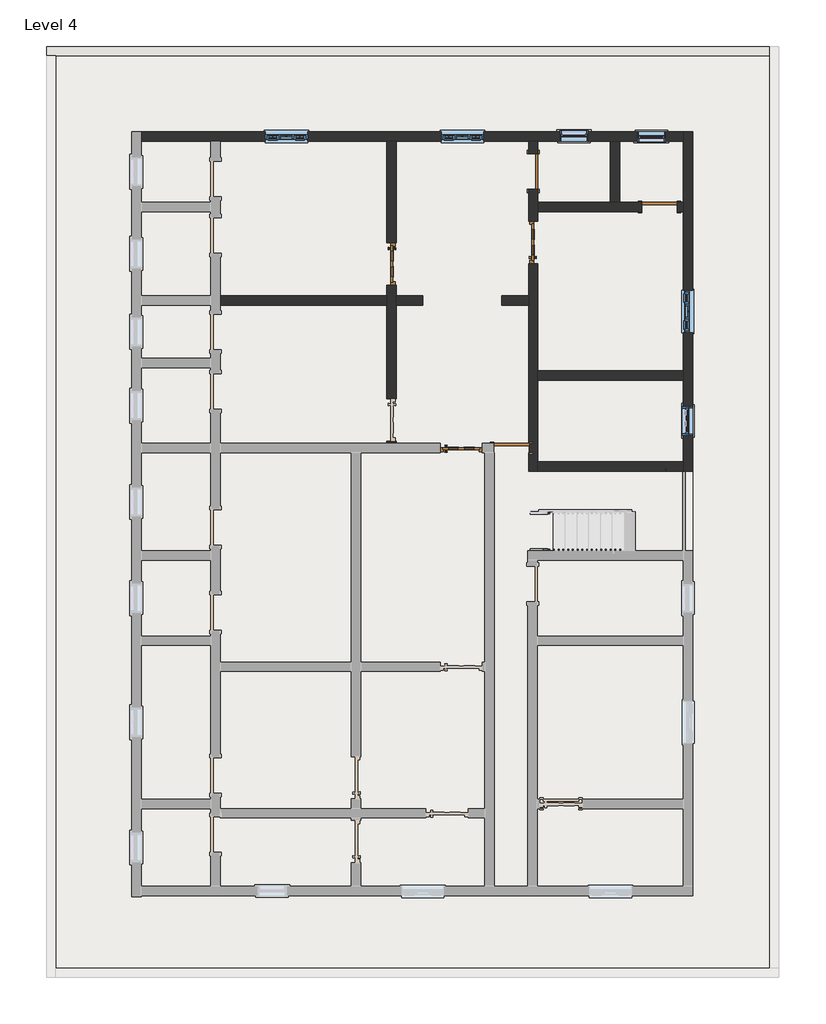
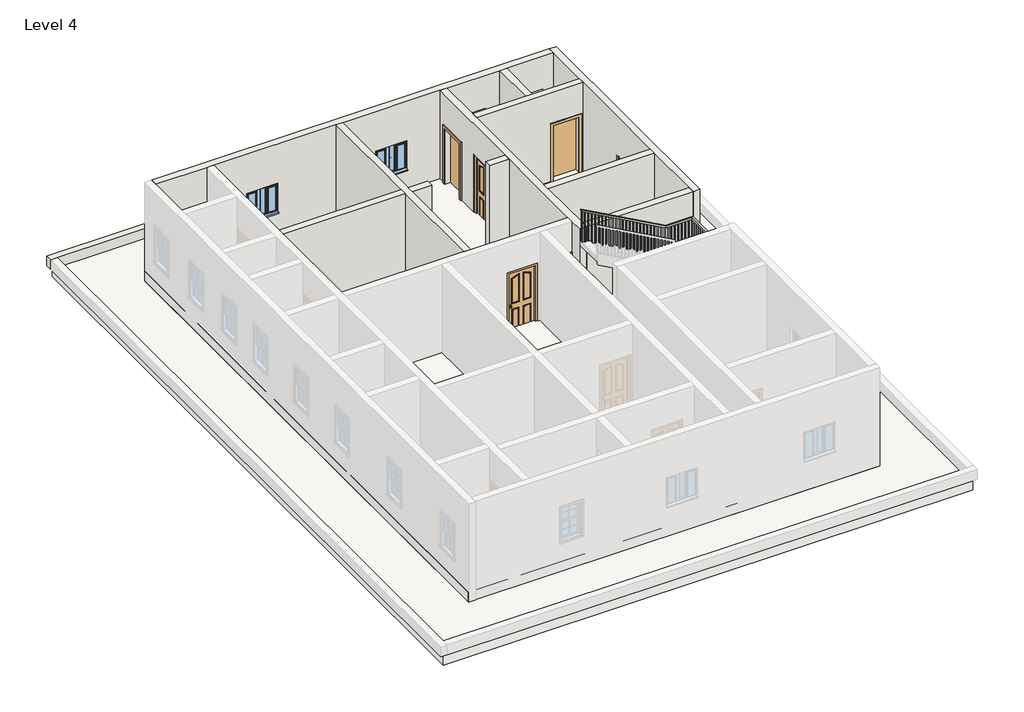
# One storey, part 2 of 3: 11 walls, 6 doors, 6 windows, 2 slabs, 1 railing, 1 roof.
"""IFC4 building model written with IfcOpenShell, lengths in millimetres."""

from ifc_helpers import new_model, si_unit, frame, origin, place, context, project, spatial, polyline, outline, extrude, faceted_brep, transform, mapped, element, save
from components import doors_extsgl_12_910x2110mm_9a09825e, doors_extsgl_12_910x2110mm_ece77ece, door_fadea3f2, window_679d2811, windows_tpl_w_glazing_cross_bars_910x910mm_4aa0f884

model = new_model("IFC4")

# Units and contexts
model_context = context("Model", 3, world=origin())
ifc_project = project(units=[si_unit("LENGTHUNIT", "METRE", prefix="MILLI")], contexts=[model_context])

# Site, building, storey
site = spatial("IfcSite", under=ifc_project)
building = spatial("IfcBuilding", under=site)
storey = spatial("IfcBuildingStorey", under=building, Name="Level 4", Elevation=9144.0)

# Doors
placement = place(None, origin())
doors_extsgl_12_910x2110mm_shape = doors_extsgl_12_910x2110mm_9a09825e(model_context)
element("IfcDoor", 1, ObjectType="Doors_ExtSgl_12 : 910x2110mm", at=placement, inside=storey, context=model_context, shape_type="MappedRepresentation", body=[
    mapped(doors_extsgl_12_910x2110mm_shape, transform((-4887.6876145, 4566.1404944, 9144.0), x_axis=(0.0, -1.0, 0.0), y_axis=(1.0, 0.0, 0.0), z_axis=(0.0, 0.0, 1.0))),
])
element("IfcDoor", 2, ObjectType="Doors_ExtSgl_12 : 910x2110mm", at=placement, inside=storey, context=model_context, shape_type="MappedRepresentation", body=[
    mapped(doors_extsgl_12_910x2110mm_shape, transform((-1839.6876145, 5029.6904944, 9144.0), x_axis=(0.0, 1.0, 0.0), y_axis=(-1.0, 0.0, 0.0), z_axis=(0.0, 0.0, 1.0))),
])
doors_extsgl_12_910x2110mm_2_shape = doors_extsgl_12_910x2110mm_ece77ece(model_context)
element("IfcDoor", 3, ObjectType="Doors_ExtSgl_12 : 910x2110mm", at=placement, inside=storey, context=model_context, shape_type="MappedRepresentation", body=[
    mapped(doors_extsgl_12_910x2110mm_2_shape, transform((-3389.0876145, 603.7404944, 9144.0), x_axis=(1.0, 0.0, 0.0), y_axis=(0.0, 1.0, 0.0), z_axis=(0.0, 0.0, 1.0))),
])
door_shape = door_fadea3f2(model_context)
element("IfcDoor", 4, ObjectType="Single-Flush : 30\" x 80\"", at=placement, inside=storey, context=model_context, shape_type="MappedRepresentation", body=[
    mapped(door_shape, transform((-1839.6876145, 6550.5154944, 9144.0), x_axis=(0.0, -1.0, 0.0), y_axis=(1.0, 0.0, 0.0), z_axis=(0.0, 0.0, 1.0))),
])
element("IfcDoor", 5, ObjectType="Single-Flush : 30\" x 80\"", at=placement, inside=storey, context=model_context, shape_type="MappedRepresentation", body=[
    mapped(door_shape, transform((878.1123855, 5791.6904944, 9144.0), x_axis=(1.0, 0.0, 0.0), y_axis=(0.0, 1.0, 0.0), z_axis=(0.0, 0.0, 1.0))),
])
element("IfcDoor", 6, ObjectType="Single-Flush : 30\" x 80\"", at=placement, inside=storey, context=model_context, shape_type="MappedRepresentation", body=[
    mapped(door_shape, transform((-2309.5876145, 603.7404944, 9144.0), x_axis=(1.0, 0.0, 0.0), y_axis=(0.0, 1.0, 0.0), z_axis=(0.0, 0.0, 1.0))),
])

# Railing
element("IfcRailing", 7, ObjectType="Handrail - Rectangular", at=placement, inside=storey, context=model_context, shape_type="SolidModel", body=[
    faceted_brep([(-1903.1876145, -1555.2595056, 10195.56), (-1903.1876145, -1555.2595056, 10137.4879132), (-1903.1876145, -1606.0595056, 10137.4879132), (-1903.1876145, -1606.0595056, 10195.56), (325.4830625, -1555.2595056, 11430.0), (338.6121628, -1555.2595056, 11379.2), (338.6121628, -1606.0595056, 11379.2), (325.4830625, -1606.0595056, 11430.0), (1322.6123855, -1555.2595056, 11430.0), (1322.6123855, -1555.2595056, 11379.2), (1373.4123855, -1606.0595056, 11379.2), (1373.4123855, -1606.0595056, 11430.0), (1322.6123855, 57.6404944, 11430.0), (1322.6123855, 57.6404944, 11379.2), (1373.4123855, 108.4404944, 11379.2), (1373.4123855, 108.4404944, 11430.0), (573.1131377, 57.6404944, 11430.0), (559.9840375, 57.6404944, 11379.2), (559.9840375, 108.4404944, 11379.2), (573.1131377, 108.4404944, 11430.0), (-1903.1876145, 57.6404944, 12801.6), (-1903.1876145, 108.4404944, 12801.6), (-1903.1876145, 108.4404944, 12743.5279132), (-1903.1876145, 57.6404944, 12743.5279132)], [[[0, 1, 2, 3]], [[1, 0, 4, 5]], [[2, 1, 5, 6]], [[3, 2, 6, 7]], [[0, 3, 7, 4]], [[5, 4, 8, 9]], [[6, 5, 9, 10]], [[7, 6, 10, 11]], [[4, 7, 11, 8]], [[9, 8, 12, 13]], [[10, 9, 13, 14]], [[11, 10, 14, 15]], [[8, 11, 15, 12]], [[13, 12, 16, 17]], [[14, 13, 17, 18]], [[15, 14, 18, 19]], [[12, 15, 19, 16]], [[20, 21, 22, 23]], [[17, 16, 20, 23]], [[18, 17, 23, 22]], [[19, 18, 22, 21]], [[16, 19, 21, 20]]]),
    extrude(outline(polyline([(12681.9768073, -1792.0626145), (12692.5284254, -1811.1126145), (11750.04, -1811.1126145), (11750.04, -1792.0626145), (12681.9768073, -1792.0626145)])), frame((0.0, 73.5154944, 0.0), z_axis=(0.0, 1.0, 0.0), x_axis=(0.0, 0.0, 1.0)), (0.0, 0.0, 1.0), 19.05),
    extrude(outline(polyline([(12625.7015104, -1690.4626145), (12636.2531286, -1709.5126145), (11750.04, -1709.5126145), (11750.04, -1690.4626145), (12625.7015104, -1690.4626145)])), frame((0.0, 73.5154944, 0.0), z_axis=(0.0, 1.0, 0.0), x_axis=(0.0, 0.0, 1.0)), (0.0, 0.0, 1.0), 19.05),
    extrude(outline(polyline([(12569.4262135, -1588.8626145), (12579.9778317, -1607.9126145), (11612.88, -1607.9126145), (11612.88, -1588.8626145), (12569.4262135, -1588.8626145)])), frame((0.0, 73.5154944, 0.0), z_axis=(0.0, 1.0, 0.0), x_axis=(0.0, 0.0, 1.0)), (0.0, 0.0, 1.0), 19.05),
    extrude(outline(polyline([(12513.1509166, -1487.2626145), (12523.7025348, -1506.3126145), (11612.88, -1506.3126145), (11612.88, -1487.2626145), (12513.1509166, -1487.2626145)])), frame((0.0, 73.5154944, 0.0), z_axis=(0.0, 1.0, 0.0), x_axis=(0.0, 0.0, 1.0)), (0.0, 0.0, 1.0), 19.05),
    extrude(outline(polyline([(12456.8756198, -1385.6626145), (12467.4272379, -1404.7126145), (11475.72, -1404.7126145), (11475.72, -1385.6626145), (12456.8756198, -1385.6626145)])), frame((0.0, 73.5154944, 0.0), z_axis=(0.0, 1.0, 0.0), x_axis=(0.0, 0.0, 1.0)), (0.0, 0.0, 1.0), 19.05),
    extrude(outline(polyline([(12400.6003229, -1284.0626145), (12411.151941, -1303.1126145), (11475.72, -1303.1126145), (11475.72, -1284.0626145), (12400.6003229, -1284.0626145)])), frame((0.0, 73.5154944, 0.0), z_axis=(0.0, 1.0, 0.0), x_axis=(0.0, 0.0, 1.0)), (0.0, 0.0, 1.0), 19.05),
    extrude(outline(polyline([(12344.325026, -1182.4626145), (12354.8766442, -1201.5126145), (11475.72, -1201.5126145), (11475.72, -1182.4626145), (12344.325026, -1182.4626145)])), frame((0.0, 73.5154944, 0.0), z_axis=(0.0, 1.0, 0.0), x_axis=(0.0, 0.0, 1.0)), (0.0, 0.0, 1.0), 19.05),
    extrude(outline(polyline([(12288.0497291, -1080.8626145), (12298.6013473, -1099.9126145), (11338.56, -1099.9126145), (11338.56, -1080.8626145), (12288.0497291, -1080.8626145)])), frame((0.0, 73.5154944, 0.0), z_axis=(0.0, 1.0, 0.0), x_axis=(0.0, 0.0, 1.0)), (0.0, 0.0, 1.0), 19.05),
    extrude(outline(polyline([(12231.7744322, -979.2626145), (12242.3260504, -998.3126145), (11338.56, -998.3126145), (11338.56, -979.2626145), (12231.7744322, -979.2626145)])), frame((0.0, 73.5154944, 0.0), z_axis=(0.0, 1.0, 0.0), x_axis=(0.0, 0.0, 1.0)), (0.0, 0.0, 1.0), 19.05),
    extrude(outline(polyline([(12175.4991354, -877.6626145), (12186.0507535, -896.7126145), (11201.4, -896.7126145), (11201.4, -877.6626145), (12175.4991354, -877.6626145)])), frame((0.0, 73.5154944, 0.0), z_axis=(0.0, 1.0, 0.0), x_axis=(0.0, 0.0, 1.0)), (0.0, 0.0, 1.0), 19.05),
    extrude(outline(polyline([(12119.2238385, -776.0626145), (12129.7754566, -795.1126145), (11201.4, -795.1126145), (11201.4, -776.0626145), (12119.2238385, -776.0626145)])), frame((0.0, 73.5154944, 0.0), z_axis=(0.0, 1.0, 0.0), x_axis=(0.0, 0.0, 1.0)), (0.0, 0.0, 1.0), 19.05),
    extrude(outline(polyline([(12062.9485416, -674.4626145), (12073.5001598, -693.5126145), (11201.4, -693.5126145), (11201.4, -674.4626145), (12062.9485416, -674.4626145)])), frame((0.0, 73.5154944, 0.0), z_axis=(0.0, 1.0, 0.0), x_axis=(0.0, 0.0, 1.0)), (0.0, 0.0, 1.0), 19.05),
    extrude(outline(polyline([(12006.6732447, -572.8626145), (12017.2248629, -591.9126145), (11064.24, -591.9126145), (11064.24, -572.8626145), (12006.6732447, -572.8626145)])), frame((0.0, 73.5154944, 0.0), z_axis=(0.0, 1.0, 0.0), x_axis=(0.0, 0.0, 1.0)), (0.0, 0.0, 1.0), 19.05),
    extrude(outline(polyline([(11950.3979478, -471.2626145), (11960.949566, -490.3126145), (11064.24, -490.3126145), (11064.24, -471.2626145), (11950.3979478, -471.2626145)])), frame((0.0, 73.5154944, 0.0), z_axis=(0.0, 1.0, 0.0), x_axis=(0.0, 0.0, 1.0)), (0.0, 0.0, 1.0), 19.05),
    extrude(outline(polyline([(11894.1226509, -369.6626145), (11904.6742691, -388.7126145), (10927.08, -388.7126145), (10927.08, -369.6626145), (11894.1226509, -369.6626145)])), frame((0.0, 73.5154944, 0.0), z_axis=(0.0, 1.0, 0.0), x_axis=(0.0, 0.0, 1.0)), (0.0, 0.0, 1.0), 19.05),
    extrude(outline(polyline([(11837.8473541, -268.0626145), (11848.3989722, -287.1126145), (10927.08, -287.1126145), (10927.08, -268.0626145), (11837.8473541, -268.0626145)])), frame((0.0, 73.5154944, 0.0), z_axis=(0.0, 1.0, 0.0), x_axis=(0.0, 0.0, 1.0)), (0.0, 0.0, 1.0), 19.05),
    extrude(outline(polyline([(11781.5720572, -166.4626145), (11792.1236754, -185.5126145), (10927.08, -185.5126145), (10927.08, -166.4626145), (11781.5720572, -166.4626145)])), frame((0.0, 73.5154944, 0.0), z_axis=(0.0, 1.0, 0.0), x_axis=(0.0, 0.0, 1.0)), (0.0, 0.0, 1.0), 19.05),
    extrude(outline(polyline([(11725.2967603, -64.8626145), (11735.8483785, -83.9126145), (10789.92, -83.9126145), (10789.92, -64.8626145), (11725.2967603, -64.8626145)])), frame((0.0, 73.5154944, 0.0), z_axis=(0.0, 1.0, 0.0), x_axis=(0.0, 0.0, 1.0)), (0.0, 0.0, 1.0), 19.05),
    extrude(outline(polyline([(11669.0214634, 36.7373855), (11679.5730816, 17.6873855), (10789.92, 17.6873855), (10789.92, 36.7373855), (11669.0214634, 36.7373855)])), frame((0.0, 73.5154944, 0.0), z_axis=(0.0, 1.0, 0.0), x_axis=(0.0, 0.0, 1.0)), (0.0, 0.0, 1.0), 19.05),
    extrude(outline(polyline([(11612.7461665, 138.3373855), (11623.2977847, 119.2873855), (10652.76, 119.2873855), (10652.76, 138.3373855), (11612.7461665, 138.3373855)])), frame((0.0, 73.5154944, 0.0), z_axis=(0.0, 1.0, 0.0), x_axis=(0.0, 0.0, 1.0)), (0.0, 0.0, 1.0), 19.05),
    extrude(outline(polyline([(11556.4708697, 239.9373855), (11567.0224878, 220.8873855), (10652.76, 220.8873855), (10652.76, 239.9373855), (11556.4708697, 239.9373855)])), frame((0.0, 73.5154944, 0.0), z_axis=(0.0, 1.0, 0.0), x_axis=(0.0, 0.0, 1.0)), (0.0, 0.0, 1.0), 19.05),
    extrude(outline(polyline([(11500.1955728, 341.5373855), (11510.7471909, 322.4873855), (10515.6, 322.4873855), (10515.6, 341.5373855), (11500.1955728, 341.5373855)])), frame((0.0, 73.5154944, 0.0), z_axis=(0.0, 1.0, 0.0), x_axis=(0.0, 0.0, 1.0)), (0.0, 0.0, 1.0), 19.05),
    extrude(outline(polyline([(11443.9202759, 443.1373855), (11454.4718941, 424.0873855), (10515.6, 424.0873855), (10515.6, 443.1373855), (11443.9202759, 443.1373855)])), frame((0.0, 73.5154944, 0.0), z_axis=(0.0, 1.0, 0.0), x_axis=(0.0, 0.0, 1.0)), (0.0, 0.0, 1.0), 19.05),
    extrude(outline(polyline([(11387.644979, 544.7373855), (11398.1965972, 525.6873855), (10515.6, 525.6873855), (10515.6, 544.7373855), (11387.644979, 544.7373855)])), frame((0.0, 73.5154944, 0.0), z_axis=(0.0, 1.0, 0.0), x_axis=(0.0, 0.0, 1.0)), (0.0, 0.0, 1.0), 19.05),
    extrude(outline(polyline([(646.3373855, 92.5654944), (646.3373855, 73.5154944), (627.2873855, 73.5154944), (627.2873855, 92.5654944), (646.3373855, 92.5654944)])), frame((0.0, 0.0, 10515.6), z_axis=(0.0, 0.0, 1.0), x_axis=(1.0, 0.0, 0.0)), (0.0, 0.0, 1.0), 863.6),
    extrude(outline(polyline([(747.9373855, 92.5654944), (747.9373855, 73.5154944), (728.8873855, 73.5154944), (728.8873855, 92.5654944), (747.9373855, 92.5654944)])), frame((0.0, 0.0, 10515.6), z_axis=(0.0, 0.0, 1.0), x_axis=(1.0, 0.0, 0.0)), (0.0, 0.0, 1.0), 863.6),
    extrude(outline(polyline([(849.5373855, 92.5654944), (849.5373855, 73.5154944), (830.4873855, 73.5154944), (830.4873855, 92.5654944), (849.5373855, 92.5654944)])), frame((0.0, 0.0, 10515.6), z_axis=(0.0, 0.0, 1.0), x_axis=(1.0, 0.0, 0.0)), (0.0, 0.0, 1.0), 863.6),
    extrude(outline(polyline([(951.1373855, 92.5654944), (951.1373855, 73.5154944), (932.0873855, 73.5154944), (932.0873855, 92.5654944), (951.1373855, 92.5654944)])), frame((0.0, 0.0, 10515.6), z_axis=(0.0, 0.0, 1.0), x_axis=(1.0, 0.0, 0.0)), (0.0, 0.0, 1.0), 863.6),
    extrude(outline(polyline([(1052.7373855, 92.5654944), (1052.7373855, 73.5154944), (1033.6873855, 73.5154944), (1033.6873855, 92.5654944), (1052.7373855, 92.5654944)])), frame((0.0, 0.0, 10515.6), z_axis=(0.0, 0.0, 1.0), x_axis=(1.0, 0.0, 0.0)), (0.0, 0.0, 1.0), 863.6),
    extrude(outline(polyline([(1154.3373855, 92.5654944), (1154.3373855, 73.5154944), (1135.2873855, 73.5154944), (1135.2873855, 92.5654944), (1154.3373855, 92.5654944)])), frame((0.0, 0.0, 10515.6), z_axis=(0.0, 0.0, 1.0), x_axis=(1.0, 0.0, 0.0)), (0.0, 0.0, 1.0), 863.6),
    extrude(outline(polyline([(1255.9373855, 92.5654944), (1255.9373855, 73.5154944), (1236.8873855, 73.5154944), (1236.8873855, 92.5654944), (1255.9373855, 92.5654944)])), frame((0.0, 0.0, 10515.6), z_axis=(0.0, 0.0, 1.0), x_axis=(1.0, 0.0, 0.0)), (0.0, 0.0, 1.0), 863.6),
    extrude(outline(polyline([(1357.5373855, 35.4154944), (1338.4873855, 35.4154944), (1338.4873855, 54.4654944), (1357.5373855, 54.4654944), (1357.5373855, 35.4154944)])), frame((0.0, 0.0, 10515.6), z_axis=(0.0, 0.0, 1.0), x_axis=(1.0, 0.0, 0.0)), (0.0, 0.0, 1.0), 863.6),
    extrude(outline(polyline([(1357.5373855, -66.1845056), (1338.4873855, -66.1845056), (1338.4873855, -47.1345056), (1357.5373855, -47.1345056), (1357.5373855, -66.1845056)])), frame((0.0, 0.0, 10515.6), z_axis=(0.0, 0.0, 1.0), x_axis=(1.0, 0.0, 0.0)), (0.0, 0.0, 1.0), 863.6),
    extrude(outline(polyline([(1357.5373855, -167.7845056), (1338.4873855, -167.7845056), (1338.4873855, -148.7345056), (1357.5373855, -148.7345056), (1357.5373855, -167.7845056)])), frame((0.0, 0.0, 10515.6), z_axis=(0.0, 0.0, 1.0), x_axis=(1.0, 0.0, 0.0)), (0.0, 0.0, 1.0), 863.6),
    extrude(outline(polyline([(1357.5373855, -269.3845056), (1338.4873855, -269.3845056), (1338.4873855, -250.3345056), (1357.5373855, -250.3345056), (1357.5373855, -269.3845056)])), frame((0.0, 0.0, 10515.6), z_axis=(0.0, 0.0, 1.0), x_axis=(1.0, 0.0, 0.0)), (0.0, 0.0, 1.0), 863.6),
    extrude(outline(polyline([(1357.5373855, -370.9845056), (1338.4873855, -370.9845056), (1338.4873855, -351.9345056), (1357.5373855, -351.9345056), (1357.5373855, -370.9845056)])), frame((0.0, 0.0, 10515.6), z_axis=(0.0, 0.0, 1.0), x_axis=(1.0, 0.0, 0.0)), (0.0, 0.0, 1.0), 863.6),
    extrude(outline(polyline([(1357.5373855, -472.5845056), (1338.4873855, -472.5845056), (1338.4873855, -453.5345056), (1357.5373855, -453.5345056), (1357.5373855, -472.5845056)])), frame((0.0, 0.0, 10515.6), z_axis=(0.0, 0.0, 1.0), x_axis=(1.0, 0.0, 0.0)), (0.0, 0.0, 1.0), 863.6),
    extrude(outline(polyline([(1357.5373855, -574.1845056), (1338.4873855, -574.1845056), (1338.4873855, -555.1345056), (1357.5373855, -555.1345056), (1357.5373855, -574.1845056)])), frame((0.0, 0.0, 10515.6), z_axis=(0.0, 0.0, 1.0), x_axis=(1.0, 0.0, 0.0)), (0.0, 0.0, 1.0), 863.6),
    extrude(outline(polyline([(1357.5373855, -675.7845056), (1338.4873855, -675.7845056), (1338.4873855, -656.7345056), (1357.5373855, -656.7345056), (1357.5373855, -675.7845056)])), frame((0.0, 0.0, 10515.6), z_axis=(0.0, 0.0, 1.0), x_axis=(1.0, 0.0, 0.0)), (0.0, 0.0, 1.0), 863.6),
    extrude(outline(polyline([(1357.5373855, -777.3845056), (1338.4873855, -777.3845056), (1338.4873855, -758.3345056), (1357.5373855, -758.3345056), (1357.5373855, -777.3845056)])), frame((0.0, 0.0, 10515.6), z_axis=(0.0, 0.0, 1.0), x_axis=(1.0, 0.0, 0.0)), (0.0, 0.0, 1.0), 863.6),
    extrude(outline(polyline([(1357.5373855, -878.9845056), (1338.4873855, -878.9845056), (1338.4873855, -859.9345056), (1357.5373855, -859.9345056), (1357.5373855, -878.9845056)])), frame((0.0, 0.0, 10515.6), z_axis=(0.0, 0.0, 1.0), x_axis=(1.0, 0.0, 0.0)), (0.0, 0.0, 1.0), 863.6),
    extrude(outline(polyline([(1357.5373855, -980.5845056), (1338.4873855, -980.5845056), (1338.4873855, -961.5345056), (1357.5373855, -961.5345056), (1357.5373855, -980.5845056)])), frame((0.0, 0.0, 10515.6), z_axis=(0.0, 0.0, 1.0), x_axis=(1.0, 0.0, 0.0)), (0.0, 0.0, 1.0), 863.6),
    extrude(outline(polyline([(1357.5373855, -1082.1845056), (1338.4873855, -1082.1845056), (1338.4873855, -1063.1345056), (1357.5373855, -1063.1345056), (1357.5373855, -1082.1845056)])), frame((0.0, 0.0, 10515.6), z_axis=(0.0, 0.0, 1.0), x_axis=(1.0, 0.0, 0.0)), (0.0, 0.0, 1.0), 863.6),
    extrude(outline(polyline([(1357.5373855, -1183.7845056), (1338.4873855, -1183.7845056), (1338.4873855, -1164.7345056), (1357.5373855, -1164.7345056), (1357.5373855, -1183.7845056)])), frame((0.0, 0.0, 10515.6), z_axis=(0.0, 0.0, 1.0), x_axis=(1.0, 0.0, 0.0)), (0.0, 0.0, 1.0), 863.6),
    extrude(outline(polyline([(1357.5373855, -1285.3845056), (1338.4873855, -1285.3845056), (1338.4873855, -1266.3345056), (1357.5373855, -1266.3345056), (1357.5373855, -1285.3845056)])), frame((0.0, 0.0, 10515.6), z_axis=(0.0, 0.0, 1.0), x_axis=(1.0, 0.0, 0.0)), (0.0, 0.0, 1.0), 863.6),
    extrude(outline(polyline([(1357.5373855, -1386.9845056), (1338.4873855, -1386.9845056), (1338.4873855, -1367.9345056), (1357.5373855, -1367.9345056), (1357.5373855, -1386.9845056)])), frame((0.0, 0.0, 10515.6), z_axis=(0.0, 0.0, 1.0), x_axis=(1.0, 0.0, 0.0)), (0.0, 0.0, 1.0), 863.6),
    extrude(outline(polyline([(1357.5373855, -1488.5845056), (1338.4873855, -1488.5845056), (1338.4873855, -1469.5345056), (1357.5373855, -1469.5345056), (1357.5373855, -1488.5845056)])), frame((0.0, 0.0, 10515.6), z_axis=(0.0, 0.0, 1.0), x_axis=(1.0, 0.0, 0.0)), (0.0, 0.0, 1.0), 863.6),
    extrude(outline(polyline([(1236.8873855, -1590.1845056), (1236.8873855, -1571.1345056), (1255.9373855, -1571.1345056), (1255.9373855, -1590.1845056), (1236.8873855, -1590.1845056)])), frame((0.0, 0.0, 10515.6), z_axis=(0.0, 0.0, 1.0), x_axis=(1.0, 0.0, 0.0)), (0.0, 0.0, 1.0), 863.6),
    extrude(outline(polyline([(1135.2873855, -1590.1845056), (1135.2873855, -1571.1345056), (1154.3373855, -1571.1345056), (1154.3373855, -1590.1845056), (1135.2873855, -1590.1845056)])), frame((0.0, 0.0, 10515.6), z_axis=(0.0, 0.0, 1.0), x_axis=(1.0, 0.0, 0.0)), (0.0, 0.0, 1.0), 863.6),
    extrude(outline(polyline([(1033.6873855, -1590.1845056), (1033.6873855, -1571.1345056), (1052.7373855, -1571.1345056), (1052.7373855, -1590.1845056), (1033.6873855, -1590.1845056)])), frame((0.0, 0.0, 10515.6), z_axis=(0.0, 0.0, 1.0), x_axis=(1.0, 0.0, 0.0)), (0.0, 0.0, 1.0), 863.6),
    extrude(outline(polyline([(932.0873855, -1590.1845056), (932.0873855, -1571.1345056), (951.1373855, -1571.1345056), (951.1373855, -1590.1845056), (932.0873855, -1590.1845056)])), frame((0.0, 0.0, 10515.6), z_axis=(0.0, 0.0, 1.0), x_axis=(1.0, 0.0, 0.0)), (0.0, 0.0, 1.0), 863.6),
    extrude(outline(polyline([(830.4873855, -1590.1845056), (830.4873855, -1571.1345056), (849.5373855, -1571.1345056), (849.5373855, -1590.1845056), (830.4873855, -1590.1845056)])), frame((0.0, 0.0, 10515.6), z_axis=(0.0, 0.0, 1.0), x_axis=(1.0, 0.0, 0.0)), (0.0, 0.0, 1.0), 863.6),
    extrude(outline(polyline([(728.8873855, -1590.1845056), (728.8873855, -1571.1345056), (747.9373855, -1571.1345056), (747.9373855, -1590.1845056), (728.8873855, -1590.1845056)])), frame((0.0, 0.0, 10515.6), z_axis=(0.0, 0.0, 1.0), x_axis=(1.0, 0.0, 0.0)), (0.0, 0.0, 1.0), 863.6),
    extrude(outline(polyline([(627.2873855, -1590.1845056), (627.2873855, -1571.1345056), (646.3373855, -1571.1345056), (646.3373855, -1590.1845056), (627.2873855, -1590.1845056)])), frame((0.0, 0.0, 10515.6), z_axis=(0.0, 0.0, 1.0), x_axis=(1.0, 0.0, 0.0)), (0.0, 0.0, 1.0), 863.6),
    extrude(outline(polyline([(525.6873855, -1590.1845056), (525.6873855, -1571.1345056), (544.7373855, -1571.1345056), (544.7373855, -1590.1845056), (525.6873855, -1590.1845056)])), frame((0.0, 0.0, 10515.6), z_axis=(0.0, 0.0, 1.0), x_axis=(1.0, 0.0, 0.0)), (0.0, 0.0, 1.0), 863.6),
    extrude(outline(polyline([(424.0873855, -1590.1845056), (424.0873855, -1571.1345056), (443.1373855, -1571.1345056), (443.1373855, -1590.1845056), (424.0873855, -1590.1845056)])), frame((0.0, 0.0, 10515.6), z_axis=(0.0, 0.0, 1.0), x_axis=(1.0, 0.0, 0.0)), (0.0, 0.0, 1.0), 863.6),
    extrude(outline(polyline([(322.4873855, -1590.1845056), (322.4873855, -1571.1345056), (341.5373855, -1571.1345056), (341.5373855, -1590.1845056), (322.4873855, -1590.1845056)])), frame((0.0, 0.0, 10515.6), z_axis=(0.0, 0.0, 1.0), x_axis=(1.0, 0.0, 0.0)), (0.0, 0.0, 1.0), 863.6),
    extrude(outline(polyline([(11324.5449568, 239.9373855), (11313.9933387, 220.8873855), (10378.44, 220.8873855), (10378.44, 239.9373855), (11324.5449568, 239.9373855)])), frame((0.0, -1590.1845056, 0.0), z_axis=(0.0, 1.0, 0.0), x_axis=(0.0, 0.0, 1.0)), (0.0, 0.0, 1.0), 19.05),
    extrude(outline(polyline([(11268.2696599, 138.3373855), (11257.7180418, 119.2873855), (10378.44, 119.2873855), (10378.44, 138.3373855), (11268.2696599, 138.3373855)])), frame((0.0, -1590.1845056, 0.0), z_axis=(0.0, 1.0, 0.0), x_axis=(0.0, 0.0, 1.0)), (0.0, 0.0, 1.0), 19.05),
    extrude(outline(polyline([(11211.9943631, 36.7373855), (11201.4427449, 17.6873855), (10241.28, 17.6873855), (10241.28, 36.7373855), (11211.9943631, 36.7373855)])), frame((0.0, -1590.1845056, 0.0), z_axis=(0.0, 1.0, 0.0), x_axis=(0.0, 0.0, 1.0)), (0.0, 0.0, 1.0), 19.05),
    extrude(outline(polyline([(11155.7190662, -64.8626145), (11145.167448, -83.9126145), (10241.28, -83.9126145), (10241.28, -64.8626145), (11155.7190662, -64.8626145)])), frame((0.0, -1590.1845056, 0.0), z_axis=(0.0, 1.0, 0.0), x_axis=(0.0, 0.0, 1.0)), (0.0, 0.0, 1.0), 19.05),
    extrude(outline(polyline([(11099.4437693, -166.4626145), (11088.8921511, -185.5126145), (10104.12, -185.5126145), (10104.12, -166.4626145), (11099.4437693, -166.4626145)])), frame((0.0, -1590.1845056, 0.0), z_axis=(0.0, 1.0, 0.0), x_axis=(0.0, 0.0, 1.0)), (0.0, 0.0, 1.0), 19.05),
    extrude(outline(polyline([(11043.1684724, -268.0626145), (11032.6168543, -287.1126145), (10104.12, -287.1126145), (10104.12, -268.0626145), (11043.1684724, -268.0626145)])), frame((0.0, -1590.1845056, 0.0), z_axis=(0.0, 1.0, 0.0), x_axis=(0.0, 0.0, 1.0)), (0.0, 0.0, 1.0), 19.05),
    extrude(outline(polyline([(10986.8931755, -369.6626145), (10976.3415574, -388.7126145), (10104.12, -388.7126145), (10104.12, -369.6626145), (10986.8931755, -369.6626145)])), frame((0.0, -1590.1845056, 0.0), z_axis=(0.0, 1.0, 0.0), x_axis=(0.0, 0.0, 1.0)), (0.0, 0.0, 1.0), 19.05),
    extrude(outline(polyline([(10930.6178787, -471.2626145), (10920.0662605, -490.3126145), (9966.96, -490.3126145), (9966.96, -471.2626145), (10930.6178787, -471.2626145)])), frame((0.0, -1590.1845056, 0.0), z_axis=(0.0, 1.0, 0.0), x_axis=(0.0, 0.0, 1.0)), (0.0, 0.0, 1.0), 19.05),
    extrude(outline(polyline([(10874.3425818, -572.8626145), (10863.7909636, -591.9126145), (9966.96, -591.9126145), (9966.96, -572.8626145), (10874.3425818, -572.8626145)])), frame((0.0, -1590.1845056, 0.0), z_axis=(0.0, 1.0, 0.0), x_axis=(0.0, 0.0, 1.0)), (0.0, 0.0, 1.0), 19.05),
    extrude(outline(polyline([(10818.0672849, -674.4626145), (10807.5156667, -693.5126145), (9829.8, -693.5126145), (9829.8, -674.4626145), (10818.0672849, -674.4626145)])), frame((0.0, -1590.1845056, 0.0), z_axis=(0.0, 1.0, 0.0), x_axis=(0.0, 0.0, 1.0)), (0.0, 0.0, 1.0), 19.05),
    extrude(outline(polyline([(10761.791988, -776.0626145), (10751.2403699, -795.1126145), (9829.8, -795.1126145), (9829.8, -776.0626145), (10761.791988, -776.0626145)])), frame((0.0, -1590.1845056, 0.0), z_axis=(0.0, 1.0, 0.0), x_axis=(0.0, 0.0, 1.0)), (0.0, 0.0, 1.0), 19.05),
    extrude(outline(polyline([(10705.5166911, -877.6626145), (10694.965073, -896.7126145), (9829.8, -896.7126145), (9829.8, -877.6626145), (10705.5166911, -877.6626145)])), frame((0.0, -1590.1845056, 0.0), z_axis=(0.0, 1.0, 0.0), x_axis=(0.0, 0.0, 1.0)), (0.0, 0.0, 1.0), 19.05),
    extrude(outline(polyline([(10649.2413943, -979.2626145), (10638.6897761, -998.3126145), (9692.64, -998.3126145), (9692.64, -979.2626145), (10649.2413943, -979.2626145)])), frame((0.0, -1590.1845056, 0.0), z_axis=(0.0, 1.0, 0.0), x_axis=(0.0, 0.0, 1.0)), (0.0, 0.0, 1.0), 19.05),
    extrude(outline(polyline([(10592.9660974, -1080.8626145), (10582.4144792, -1099.9126145), (9692.64, -1099.9126145), (9692.64, -1080.8626145), (10592.9660974, -1080.8626145)])), frame((0.0, -1590.1845056, 0.0), z_axis=(0.0, 1.0, 0.0), x_axis=(0.0, 0.0, 1.0)), (0.0, 0.0, 1.0), 19.05),
    extrude(outline(polyline([(10536.6908005, -1182.4626145), (10526.1391823, -1201.5126145), (9555.48, -1201.5126145), (9555.48, -1182.4626145), (10536.6908005, -1182.4626145)])), frame((0.0, -1590.1845056, 0.0), z_axis=(0.0, 1.0, 0.0), x_axis=(0.0, 0.0, 1.0)), (0.0, 0.0, 1.0), 19.05),
    extrude(outline(polyline([(10480.4155036, -1284.0626145), (10469.8638855, -1303.1126145), (9555.48, -1303.1126145), (9555.48, -1284.0626145), (10480.4155036, -1284.0626145)])), frame((0.0, -1590.1845056, 0.0), z_axis=(0.0, 1.0, 0.0), x_axis=(0.0, 0.0, 1.0)), (0.0, 0.0, 1.0), 19.05),
    extrude(outline(polyline([(10424.1402067, -1385.6626145), (10413.5885886, -1404.7126145), (9555.48, -1404.7126145), (9555.48, -1385.6626145), (10424.1402067, -1385.6626145)])), frame((0.0, -1590.1845056, 0.0), z_axis=(0.0, 1.0, 0.0), x_axis=(0.0, 0.0, 1.0)), (0.0, 0.0, 1.0), 19.05),
    extrude(outline(polyline([(10367.8649099, -1487.2626145), (10357.3132917, -1506.3126145), (9418.32, -1506.3126145), (9418.32, -1487.2626145), (10367.8649099, -1487.2626145)])), frame((0.0, -1590.1845056, 0.0), z_axis=(0.0, 1.0, 0.0), x_axis=(0.0, 0.0, 1.0)), (0.0, 0.0, 1.0), 19.05),
    extrude(outline(polyline([(10311.589613, -1588.8626145), (10301.0379948, -1607.9126145), (9418.32, -1607.9126145), (9418.32, -1588.8626145), (10311.589613, -1588.8626145)])), frame((0.0, -1590.1845056, 0.0), z_axis=(0.0, 1.0, 0.0), x_axis=(0.0, 0.0, 1.0)), (0.0, 0.0, 1.0), 19.05),
    extrude(outline(polyline([(10255.3143161, -1690.4626145), (10244.7626979, -1709.5126145), (9281.16, -1709.5126145), (9281.16, -1690.4626145), (10255.3143161, -1690.4626145)])), frame((0.0, -1590.1845056, 0.0), z_axis=(0.0, 1.0, 0.0), x_axis=(0.0, 0.0, 1.0)), (0.0, 0.0, 1.0), 19.05),
    extrude(outline(polyline([(10199.0390192, -1792.0626145), (10188.487401, -1811.1126145), (9281.16, -1811.1126145), (9281.16, -1792.0626145), (10199.0390192, -1792.0626145)])), frame((0.0, -1590.1845056, 0.0), z_axis=(0.0, 1.0, 0.0), x_axis=(0.0, 0.0, 1.0)), (0.0, 0.0, 1.0), 19.05),
    extrude(outline(polyline([(1357.5373855, 73.5154944), (1338.4873855, 73.5154944), (1338.4873855, 92.5654944), (1357.5373855, 92.5654944), (1357.5373855, 73.5154944)])), frame((0.0, 0.0, 10515.6), z_axis=(0.0, 0.0, 1.0), x_axis=(1.0, 0.0, 0.0)), (0.0, 0.0, 1.0), 863.6),
    extrude(outline(polyline([(1338.4873855, -1590.1845056), (1338.4873855, -1571.1345056), (1357.5373855, -1571.1345056), (1357.5373855, -1590.1845056), (1338.4873855, -1590.1845056)])), frame((0.0, 0.0, 10515.6), z_axis=(0.0, 0.0, 1.0), x_axis=(1.0, 0.0, 0.0)), (0.0, 0.0, 1.0), 863.6),
    extrude(outline(polyline([(12732.9762951, -1884.1376145), (12743.5279132, -1903.1876145), (11750.04, -1903.1876145), (11750.04, -1884.1376145), (12732.9762951, -1884.1376145)])), frame((0.0, 73.5154944, 0.0), z_axis=(0.0, 1.0, 0.0), x_axis=(0.0, 0.0, 1.0)), (0.0, 0.0, 1.0), 19.05),
    extrude(outline(polyline([(10148.0395314, -1884.1376145), (10137.4879132, -1903.1876145), (9281.16, -1903.1876145), (9281.16, -1884.1376145), (10148.0395314, -1884.1376145)])), frame((0.0, -1590.1845056, 0.0), z_axis=(0.0, 1.0, 0.0), x_axis=(0.0, 0.0, 1.0)), (0.0, 0.0, 1.0), 19.05),
])

# Roof
element("IfcRoof", 8, ObjectType="Generic - 12\"", at=placement, inside=storey, context=model_context, shape_type="SweptSolid", body=[
    extrude(outline(polyline([(-10475.6876145, 7410.9404944), (1589.3123855, 7410.9404944), (1589.3123855, -9022.8595056), (-10475.6876145, -9022.8595056), (-10475.6876145, 7410.9404944)])), frame((0.0, 0.0, 9144.0), z_axis=(0.0, 0.0, 1.0), x_axis=(1.0, 0.0, 0.0)), (0.0, 0.0, 1.0), 304.8),
])

# Slabs
element("IfcSlab", 9, ObjectType="Generic - 12\"", at=placement, inside=storey, context=model_context, shape_type="SweptSolid", body=[
    extrude(outline(polyline([(1589.3123855, 7410.9404944), (1589.3123855, -9022.8595056), (-10475.6876145, -9022.8595056), (-10475.6876145, 7410.9404944), (1589.3123855, 7410.9404944)])), frame((0.0, 0.0, 8839.2), z_axis=(0.0, 0.0, 1.0), x_axis=(1.0, 0.0, 0.0)), (0.0, 0.0, 1.0), 304.8),
])
element("IfcSlab", 10, ObjectType="Generic - 12\"", at=placement, inside=storey, context=model_context, shape_type="SweptSolid", body=[
    extrude(outline(polyline([(3316.5123855, 9138.1404944), (3316.5123855, -10750.0595056), (-12202.8876145, -10750.0595056), (-12202.8876145, 9138.1404944), (3316.5123855, 9138.1404944)])), frame((0.0, 0.0, 8839.2), z_axis=(0.0, 0.0, 1.0), x_axis=(1.0, 0.0, 0.0)), (0.0, 0.0, 1.0), 304.8),
])

# Walls
element("IfcWall", 11, ObjectType="4.5\"", at=placement, inside=storey, context=model_context, shape_type="Brep", body=[
    faceted_brep([(-4989.2876145, 758.3404944, 11254.0), (-4989.2876145, 758.3404944, 9144.0), (-4989.2876145, 705.3404944, 9144.0), (-4989.2876145, 705.3404944, 12192.0), (-4989.2876145, 3677.1404944, 12192.0), (-4989.2876145, 3880.3404944, 12192.0), (-4989.2876145, 7207.7404944, 12192.0), (-4989.2876145, 7207.7404944, 9144.0), (-4989.2876145, 5021.1404944, 9144.0), (-4989.2876145, 5021.1404944, 11254.0), (-4989.2876145, 4111.1404944, 11254.0), (-4989.2876145, 4111.1404944, 9144.0), (-4989.2876145, 3880.3404944, 9144.0), (-4989.2876145, 3677.1404944, 9144.0), (-4989.2876145, 1668.3404944, 9144.0), (-4989.2876145, 1668.3404944, 11254.0), (-4786.0876145, 705.3404944, 9144.0), (-4786.0876145, 758.3404944, 9144.0), (-4786.0876145, 758.3404944, 11254.0), (-4786.0876145, 1668.3404944, 11254.0), (-4786.0876145, 1668.3404944, 9144.0), (-4786.0876145, 3677.1404944, 9144.0), (-4786.0876145, 3880.3404944, 9144.0), (-4786.0876145, 4111.1404944, 9144.0), (-4786.0876145, 4111.1404944, 11254.0), (-4786.0876145, 5021.1404944, 11254.0), (-4786.0876145, 5021.1404944, 9144.0), (-4786.0876145, 7207.7404944, 9144.0), (-4786.0876145, 7207.7404944, 12192.0), (-4786.0876145, 3880.3404944, 12192.0), (-4786.0876145, 3677.1404944, 12192.0), (-4786.0876145, 705.3404944, 12192.0)], [[[0, 1, 2, 3, 4, 5, 6, 7, 8, 9, 10, 11, 12, 13, 14, 15]], [[16, 17, 18, 19, 20, 21, 22, 23, 24, 25, 26, 27, 28, 29, 30, 31]], [[8, 7, 27, 26]], [[2, 1, 17, 16]], [[14, 13, 12, 11, 23, 22, 21, 20]], [[6, 5, 4, 3, 31, 30, 29, 28]], [[7, 6, 28, 27]], [[3, 2, 16, 31]], [[26, 25, 9, 8]], [[24, 23, 11, 10]], [[25, 24, 10, 9]], [[20, 19, 15, 14]], [[18, 17, 1, 0]], [[19, 18, 0, 15]]]),
])
element("IfcWall", 12, ObjectType="4.5\"", at=placement, inside=storey, context=model_context, shape_type="SweptSolid", body=[
    extrude(outline(polyline([(-4214.5876145, 3880.3404944), (-4214.5876145, 3677.1404944), (-4786.0876145, 3677.1404944), (-4786.0876145, 3880.3404944), (-4214.5876145, 3880.3404944)])), frame((0.0, 0.0, 9144.0), z_axis=(0.0, 0.0, 1.0), x_axis=(1.0, 0.0, 0.0)), (0.0, 0.0, 1.0), 3048.0),
    extrude(outline(polyline([(-8570.6876145, 3677.1404944), (-8570.6876145, 3880.3404944), (-4989.2876145, 3880.3404944), (-4989.2876145, 3677.1404944), (-8570.6876145, 3677.1404944)])), frame((0.0, 0.0, 9144.0), z_axis=(0.0, 0.0, 1.0), x_axis=(1.0, 0.0, 0.0)), (0.0, 0.0, 1.0), 3048.0),
])
element("IfcWall", 13, ObjectType="4.5\"", at=placement, inside=storey, context=model_context, shape_type="Brep", body=[
    faceted_brep([(-1941.2876145, 6169.5154944, 9144.0), (-1941.2876145, 5484.6904944, 9144.0), (-1941.2876145, 5484.6904944, 11254.0), (-1941.2876145, 4574.6904944, 11254.0), (-1941.2876145, 4574.6904944, 9144.0), (-1941.2876145, 3880.3404944, 9144.0), (-1941.2876145, 3677.1404944, 9144.0), (-1941.2876145, 705.3404944, 9144.0), (-1941.2876145, 705.3404944, 11176.0), (-1941.2876145, 502.1404944, 11176.0), (-1941.2876145, 502.1404944, 9144.0), (-1941.2876145, 108.4404944, 9144.0), (-1941.2876145, 108.4404944, 12192.0), (-1941.2876145, 502.1404944, 12192.0), (-1941.2876145, 705.3404944, 12192.0), (-1941.2876145, 3677.1404944, 12192.0), (-1941.2876145, 3880.3404944, 12192.0), (-1941.2876145, 7207.7404944, 12192.0), (-1941.2876145, 7207.7404944, 9144.0), (-1941.2876145, 6931.5154944, 9144.0), (-1941.2876145, 6931.5154944, 11176.0), (-1941.2876145, 6169.5154944, 11176.0), (-1738.0876145, 5484.6904944, 11254.0), (-1738.0876145, 5484.6904944, 9144.0), (-1738.0876145, 5690.0904944, 9144.0), (-1738.0876145, 5893.2904944, 9144.0), (-1738.0876145, 6169.5154944, 9144.0), (-1738.0876145, 6169.5154944, 11176.0), (-1738.0876145, 6931.5154944, 11176.0), (-1738.0876145, 6931.5154944, 9144.0), (-1738.0876145, 7207.7404944, 9144.0), (-1738.0876145, 7207.7404944, 12192.0), (-1738.0876145, 5893.2904944, 12192.0), (-1738.0876145, 5690.0904944, 12192.0), (-1738.0876145, 2272.4885783, 12192.0), (-1738.0876145, 2069.2885783, 12192.0), (-1738.0876145, 311.6404944, 12192.0), (-1738.0876145, 108.4404944, 12192.0), (-1738.0876145, 108.4404944, 9144.0), (-1738.0876145, 311.6404944, 9144.0), (-1738.0876145, 2069.2885783, 9144.0), (-1738.0876145, 2272.4885783, 9144.0), (-1738.0876145, 4574.6904944, 9144.0), (-1738.0876145, 4574.6904944, 11254.0), (-1928.5876145, 502.1404944, 9144.0), (-1928.5876145, 705.3404944, 9144.0), (-1928.5876145, 502.1404944, 11176.0), (-1928.5876145, 705.3404944, 11176.0)], [[[0, 1, 2, 3, 4, 5, 6, 7, 8, 9, 10, 11, 12, 13, 14, 15, 16, 17, 18, 19, 20, 21]], [[22, 23, 24, 25, 26, 27, 28, 29, 30, 31, 32, 33, 34, 35, 36, 37, 38, 39, 40, 41, 42, 43]], [[18, 30, 29, 19]], [[42, 41, 40, 39, 38, 11, 10, 44, 45, 7, 6, 5, 4]], [[26, 25, 24, 23, 1, 0]], [[17, 16, 15, 14, 13, 12, 37, 36, 35, 34, 33, 32, 31]], [[18, 17, 31, 30]], [[12, 11, 38, 37]], [[27, 26, 0, 21]], [[28, 27, 21, 20]], [[29, 28, 20, 19]], [[46, 44, 10, 9]], [[45, 47, 8, 7]], [[44, 46, 47, 45]], [[47, 46, 9, 8]], [[4, 3, 43, 42]], [[2, 1, 23, 22]], [[3, 2, 22, 43]]]),
])
element("IfcWall", 14, ObjectType="4.5\"", at=placement, inside=storey, context=model_context, shape_type="SweptSolid", body=[
    extrude(outline(polyline([(-2512.7876145, 3880.3404944), (-1941.2876145, 3880.3404944), (-1941.2876145, 3677.1404944), (-2512.7876145, 3677.1404944), (-2512.7876145, 3880.3404944)])), frame((0.0, 0.0, 9144.0), z_axis=(0.0, 0.0, 1.0), x_axis=(1.0, 0.0, 0.0)), (0.0, 0.0, 1.0), 3048.0),
])
element("IfcWall", 15, ObjectType="4.5\"", at=placement, inside=storey, context=model_context, shape_type="SweptSolid", body=[
    extrude(outline(polyline([(1386.1123855, 108.4404944), (-1738.0876145, 108.4404944), (-1738.0876145, 311.6404944), (1386.1123855, 311.6404944), (1386.1123855, 108.4404944)])), frame((0.0, 0.0, 9144.0), z_axis=(0.0, 0.0, 1.0), x_axis=(1.0, 0.0, 0.0)), (0.0, 0.0, 1.0), 3048.0),
])
element("IfcWall", 16, ObjectType="4.5\"", at=placement, inside=storey, context=model_context, shape_type="SweptSolid", body=[
    extrude(outline(polyline([(1386.1123855, 2069.2885783), (-1738.0876145, 2069.2885783), (-1738.0876145, 2272.4885783), (1386.1123855, 2272.4885783), (1386.1123855, 2069.2885783)])), frame((0.0, 0.0, 9144.0), z_axis=(0.0, 0.0, 1.0), x_axis=(1.0, 0.0, 0.0)), (0.0, 0.0, 1.0), 3048.0),
])
element("IfcWall", 17, ObjectType="4.5\"", at=placement, inside=storey, context=model_context, shape_type="Brep", body=[
    faceted_brep([(1259.1123855, 5690.0904944, 11176.0), (1259.1123855, 5690.0904944, 9144.0), (1386.1123855, 5690.0904944, 9144.0), (1386.1123855, 5690.0904944, 12192.0), (-1738.0876145, 5690.0904944, 12192.0), (-1738.0876145, 5690.0904944, 9144.0), (497.1123855, 5690.0904944, 9144.0), (497.1123855, 5690.0904944, 11176.0), (1386.1123855, 5893.2904944, 9144.0), (1259.1123855, 5893.2904944, 9144.0), (1259.1123855, 5893.2904944, 11176.0), (497.1123855, 5893.2904944, 11176.0), (497.1123855, 5893.2904944, 9144.0), (14.5123855, 5893.2904944, 9144.0), (-188.6876145, 5893.2904944, 9144.0), (-1738.0876145, 5893.2904944, 9144.0), (-1738.0876145, 5893.2904944, 12192.0), (-188.6876145, 5893.2904944, 12192.0), (14.5123855, 5893.2904944, 12192.0), (1386.1123855, 5893.2904944, 12192.0)], [[[0, 1, 2, 3, 4, 5, 6, 7]], [[8, 9, 10, 11, 12, 13, 14, 15, 16, 17, 18, 19]], [[6, 5, 15, 14, 13, 12]], [[2, 1, 9, 8]], [[4, 3, 19, 18, 17, 16]], [[3, 2, 8, 19]], [[5, 4, 16, 15]], [[10, 9, 1, 0]], [[11, 10, 0, 7]], [[12, 11, 7, 6]]]),
])
element("IfcWall", 18, ObjectType="4.5\"", at=placement, inside=storey, context=model_context, shape_type="SweptSolid", body=[
    extrude(outline(polyline([(-188.6876145, 5893.2904944), (-188.6876145, 7207.7404944), (14.5123855, 7207.7404944), (14.5123855, 5893.2904944), (-188.6876145, 5893.2904944)])), frame((0.0, 0.0, 9144.0), z_axis=(0.0, 0.0, 1.0), x_axis=(1.0, 0.0, 0.0)), (0.0, 0.0, 1.0), 3048.0),
])
element("IfcWall", 19, ObjectType="4.5\"", at=placement, inside=storey, context=model_context, shape_type="Brep", body=[
    faceted_brep([(-12304.4876145, 9036.5404944, 9144.0), (-12101.2876145, 9036.5404944, 9144.0), (3240.3123855, 9036.5404944, 9144.0), (3240.3123855, 9036.5404944, 9448.8), (-12101.2876145, 9036.5404944, 9448.8), (-12304.4876145, 9036.5404944, 9448.8), (-12304.4876145, 9239.7404944, 9144.0), (-12304.4876145, 9239.7404944, 9448.8), (3240.3123855, 9239.7404944, 9448.8), (3240.3123855, 9239.7404944, 9144.0)], [[[0, 1, 2, 3, 4, 5]], [[6, 7, 8, 9]], [[2, 1, 0, 6, 9]], [[5, 4, 3, 8, 7]], [[0, 5, 7, 6]], [[3, 2, 9, 8]]]),
])
element("IfcWall", 20, ObjectType="Generic - 9\"", at=placement, inside=storey, context=model_context, shape_type="Brep", body=[
    faceted_brep([(1386.1123855, 7410.9404944, 9144.0), (1386.1123855, 7207.7404944, 9144.0), (1386.1123855, 5893.2904944, 9144.0), (1386.1123855, 5690.0904944, 9144.0), (1386.1123855, 2272.4885783, 9144.0), (1386.1123855, 2069.2885783, 9144.0), (1386.1123855, 311.6404944, 9144.0), (1386.1123855, 108.4404944, 9144.0), (1386.1123855, 108.4404944, 12192.0), (1386.1123855, 311.6404944, 12192.0), (1386.1123855, 2069.2885783, 12192.0), (1386.1123855, 2272.4885783, 12192.0), (1386.1123855, 5690.0904944, 12192.0), (1386.1123855, 5893.2904944, 12192.0), (1386.1123855, 7207.7404944, 12192.0), (1386.1123855, 7410.9404944, 12192.0), (1386.1123855, 3087.4885783, 10968.4), (1386.1123855, 3087.4885783, 10058.4), (1386.1123855, 3997.4885783, 10058.4), (1386.1123855, 3997.4885783, 10968.4), (1386.1123855, 885.6645364, 11125.2), (1386.1123855, 885.6645364, 10058.4), (1386.1123855, 1495.2645364, 10058.4), (1386.1123855, 1495.2645364, 11125.2), (1589.3123855, 7410.9404944, 9144.0), (1589.3123855, 7410.9404944, 12192.0), (1589.3123855, 108.4404944, 12192.0), (1589.3123855, 108.4404944, 9144.0), (1589.3123855, 3087.4885783, 10968.4), (1589.3123855, 3997.4885783, 10968.4), (1589.3123855, 3997.4885783, 10058.4), (1589.3123855, 3087.4885783, 10058.4), (1589.3123855, 885.6645364, 11125.2), (1589.3123855, 1495.2645364, 11125.2), (1589.3123855, 1495.2645364, 10058.4), (1589.3123855, 885.6645364, 10058.4)], [[[0, 1, 2, 3, 4, 5, 6, 7, 8, 9, 10, 11, 12, 13, 14, 15], [16, 17, 18, 19], [20, 21, 22, 23]], [[24, 25, 26, 27], [28, 29, 30, 31], [32, 33, 34, 35]], [[7, 6, 5, 4, 3, 2, 1, 0, 24, 27]], [[15, 14, 13, 12, 11, 10, 9, 8, 26, 25]], [[0, 15, 25, 24]], [[8, 7, 27, 26]], [[17, 16, 28, 31]], [[18, 17, 31, 30]], [[19, 18, 30, 29]], [[16, 19, 29, 28]], [[21, 20, 32, 35]], [[22, 21, 35, 34]], [[23, 22, 34, 33]], [[20, 23, 33, 32]]]),
])
element("IfcWall", 21, ObjectType="Generic - 9\"", at=placement, inside=storey, context=model_context, shape_type="Brep", body=[
    faceted_brep([(-10272.4876145, 7207.7404944, 9144.0), (-8773.8876145, 7207.7404944, 9144.0), (-8570.6876145, 7207.7404944, 9144.0), (-4989.2876145, 7207.7404944, 9144.0), (-4786.0876145, 7207.7404944, 9144.0), (-1941.2876145, 7207.7404944, 9144.0), (-1738.0876145, 7207.7404944, 9144.0), (-188.6876145, 7207.7404944, 9144.0), (14.5123855, 7207.7404944, 9144.0), (1386.1123855, 7207.7404944, 9144.0), (1386.1123855, 7207.7404944, 12192.0), (14.5123855, 7207.7404944, 12192.0), (-188.6876145, 7207.7404944, 12192.0), (-1738.0876145, 7207.7404944, 12192.0), (-1941.2876145, 7207.7404944, 12192.0), (-4786.0876145, 7207.7404944, 12192.0), (-4989.2876145, 7207.7404944, 12192.0), (-8570.6876145, 7207.7404944, 12192.0), (-8773.8876145, 7207.7404944, 12192.0), (-10272.4876145, 7207.7404944, 12192.0), (-6693.2876145, 7207.7404944, 10968.4), (-6693.2876145, 7207.7404944, 10058.4), (-7603.2876145, 7207.7404944, 10058.4), (-7603.2876145, 7207.7404944, 10968.4), (1005.1123855, 7207.7404944, 11125.2), (1005.1123855, 7207.7404944, 10058.4), (395.5123855, 7207.7404944, 10058.4), (395.5123855, 7207.7404944, 11125.2), (-1268.1876145, 7207.7404944, 11125.2), (-658.5876145, 7207.7404944, 11125.2), (-658.5876145, 7207.7404944, 10058.4), (-1268.1876145, 7207.7404944, 10058.4), (-2908.6876145, 7207.7404944, 10968.4), (-2908.6876145, 7207.7404944, 10058.4), (-3818.6876145, 7207.7404944, 10058.4), (-3818.6876145, 7207.7404944, 10968.4), (-10272.4876145, 7410.9404944, 9144.0), (-10272.4876145, 7410.9404944, 12192.0), (1386.1123855, 7410.9404944, 12192.0), (1386.1123855, 7410.9404944, 9144.0), (-6693.2876145, 7410.9404944, 10968.4), (-7603.2876145, 7410.9404944, 10968.4), (-7603.2876145, 7410.9404944, 10058.4), (-6693.2876145, 7410.9404944, 10058.4), (1005.1123855, 7410.9404944, 11125.2), (395.5123855, 7410.9404944, 11125.2), (395.5123855, 7410.9404944, 10058.4), (1005.1123855, 7410.9404944, 10058.4), (-1268.1876145, 7410.9404944, 11125.2), (-1268.1876145, 7410.9404944, 10058.4), (-658.5876145, 7410.9404944, 10058.4), (-658.5876145, 7410.9404944, 11125.2), (-2908.6876145, 7410.9404944, 10968.4), (-3818.6876145, 7410.9404944, 10968.4), (-3818.6876145, 7410.9404944, 10058.4), (-2908.6876145, 7410.9404944, 10058.4)], [[[0, 1, 2, 3, 4, 5, 6, 7, 8, 9, 10, 11, 12, 13, 14, 15, 16, 17, 18, 19], [20, 21, 22, 23], [24, 25, 26, 27], [28, 29, 30, 31], [32, 33, 34, 35]], [[36, 37, 38, 39], [40, 41, 42, 43], [44, 45, 46, 47], [48, 49, 50, 51], [52, 53, 54, 55]], [[9, 8, 7, 6, 5, 4, 3, 2, 1, 0, 36, 39]], [[19, 18, 17, 16, 15, 14, 13, 12, 11, 10, 38, 37]], [[10, 9, 39, 38]], [[0, 19, 37, 36]], [[21, 20, 40, 43]], [[22, 21, 43, 42]], [[23, 22, 42, 41]], [[20, 23, 41, 40]], [[25, 24, 44, 47]], [[26, 25, 47, 46]], [[27, 26, 46, 45]], [[24, 27, 45, 44]], [[49, 48, 28, 31]], [[50, 49, 31, 30]], [[51, 50, 30, 29]], [[48, 51, 29, 28]], [[33, 32, 52, 55]], [[34, 33, 55, 54]], [[35, 34, 54, 53]], [[32, 35, 53, 52]]]),
])

# Windows
window_shape = window_679d2811(model_context)
element("IfcWindow", 22, ObjectType="Window-Double-Hung : 24\" x 42\"", at=placement, inside=storey, context=model_context, shape_type="MappedRepresentation", body=[
    mapped(window_shape, transform((1487.7123855, 1190.4645364, 9144.0), x_axis=(0.0, 1.0, 0.0), y_axis=(-1.0, 0.0, 0.0), z_axis=(0.0, 0.0, 1.0))),
])
element("IfcWindow", 23, ObjectType="Window-Double-Hung : 24\" x 42\"", at=placement, inside=storey, context=model_context, shape_type="MappedRepresentation", body=[
    mapped(window_shape, transform((700.3123855, 7309.3404944, 9144.0), x_axis=(-1.0, 0.0, 0.0), y_axis=(0.0, -1.0, 0.0), z_axis=(0.0, 0.0, 1.0))),
])
element("IfcWindow", 24, ObjectType="Window-Double-Hung : 24\" x 42\"", at=placement, inside=storey, context=model_context, shape_type="MappedRepresentation", body=[
    mapped(window_shape, transform((-963.3876145, 7309.3404944, 9144.0), x_axis=(1.0, 0.0, 0.0), y_axis=(0.0, 1.0, 0.0), z_axis=(0.0, 0.0, 1.0))),
])
windows_tpl_w_glazing_cross_bars_910x910mm_shape = windows_tpl_w_glazing_cross_bars_910x910mm_4aa0f884(model_context)
element("IfcWindow", 25, ObjectType="Windows_Tpl_w-Glazing_Cross-Bars : 910x910mm", at=placement, inside=storey, context=model_context, shape_type="MappedRepresentation", body=[
    mapped(windows_tpl_w_glazing_cross_bars_910x910mm_shape, transform((1496.1689533, 3969.155245, 8858.4), x_axis=(0.0, 1.0, 0.0), y_axis=(-1.0, 0.0, 0.0), z_axis=(0.0, 0.0, 1.0))),
])
element("IfcWindow", 26, ObjectType="Windows_Tpl_w-Glazing_Cross-Bars : 910x910mm", at=placement, inside=storey, context=model_context, shape_type="MappedRepresentation", body=[
    mapped(windows_tpl_w_glazing_cross_bars_910x910mm_shape, transform((-7574.9542812, 7317.7970622, 8858.4), x_axis=(-1.0, 0.0, 0.0), y_axis=(0.0, -1.0, 0.0), z_axis=(0.0, 0.0, 1.0))),
])
element("IfcWindow", 27, ObjectType="Windows_Tpl_w-Glazing_Cross-Bars : 910x910mm", at=placement, inside=storey, context=model_context, shape_type="MappedRepresentation", body=[
    mapped(windows_tpl_w_glazing_cross_bars_910x910mm_shape, transform((-3790.3542812, 7317.7970622, 8858.4), x_axis=(-1.0, 0.0, 0.0), y_axis=(0.0, -1.0, 0.0), z_axis=(0.0, 0.0, 1.0))),
])

save(model, "model.ifc")

# Revit data of these elements
# Type "Doors_ExtSgl_12 : 910x2110mm"
#   Type Mark = "8"
#   Type Comments = "External Single"
#   Operation = "SingleSwingRight"
#   Construction Type Id = "SGL"
#   Keynote = "L20"
#   Analytic Construction = "Large single-glazed windows"
#   Wrap Layers (Int) from Ext = 0' - 6.98819"
#   Wrap Layers (Ext) from Ext = 0' - 4.03543"
#   Visual Light Transmittance = 0.9
#   Thickness = 0' - 1.73228"
#   Stile Top of Lock rail = 3' - 3.37008"
#   Stile Top Rail = 0' - 5.90551"
#   Stile Shutting = 0' - 4.92126"
#   Stile Muntin Rail = 0' - 4.92126"
#   Stile Lock Rail = 0' - 6.88976"
#   Stile Hanging = 0' - 4.92126"
#   Stile Bottom Rail = 0' - 6.88976"
#   Solar Heat Gain Coefficient = 0.86
#   Rough Width = 2' - 11.82677"
#   Rough Height = 6' - 11.07087"
#   O/A Frame Width = 0' - 2.51969"
#   Heat Transfer Coefficient (U) = 0.979472 BTU/(h·ft²·°F)
#   Handle Z Distance = 3' - 3.37008"
#   Glazing Thickness = 0' - 0.94488"
#   FrameWidth = 0' - 1.65354"
#   FrameOffset - External = 0' - 0.98425"
#   FrameDepth = 0' - 3.50394"
#   Door Panel Width = 2' - 7.77165"
#   Door Panel Thickness = 0' - 1.73228"
#   Door Panel Height = 6' - 6.74016"
#   Cill Thickness = 0' - 2.14567"
#   Cill Projection = 0' - 1.1811"
#   Handle X Distance = 0' - 2.95276"
#   Height = 6' - 11.07087"
#   Structural Tolerance = 0' - 0.25591"
#   Tolerance = 0' - 0.11811"
#   Undercut = 0' - 0.15748"
#   Width = 2' - 11.82677"
#   Cill Extension = 0' - 0.98425"
#   Cavity Closer Width = 0' - 1.9685"
#   Cavity Closer Offset from Ext = 0' - 4.03543"
#   Cavity Closer Depth = 0' - 3.34646"
#   Vis - Ironmongery = yes
#   Vis - Cavity Closers = yes
#   Define Thermal Properties by = 1
#   Function = 1
#   Material Glass = Door - Glazing
#   Material Door = Door - Panel
#   Material Frame = Door - Frame/Mullion
#   Material Ironmongery = Door - Handle
#   Wall Closure = (empty or 0)
# Type "Single-Flush : 30\" x 80\""
#   Type Mark = "5"
#   Construction Type Id = "MDOOR"
#   Assembly Code = "C1020"
#   Analytic Construction = "Metal"
#   Thickness = 0' - 2"
#   Heat Transfer Coefficient (U) = 0.651978 BTU/(h·ft²·°F)
#   Height = 6' - 8"
#   Trim Projection Ext = 0' - 1"
#   Trim Projection Int = 0' - 1"
#   Trim Width = 0' - 3"
#   Width = 2' - 6"
#   Define Thermal Properties by = 1
#   Define Thermal Properties by = 1
#   Door Material = Door - Panel
#   Frame Material = Door - Frame
#   Visual Light Transmittance = 0
#   Solar Heat Gain Coefficient = 0
#   Function = (empty or 0)
#   Wall Closure = (empty or 0)
# Type "Handrail - Rectangular"
#   Assembly Code = "C2010400"
#   built-in parameter 1008612 = 0.0416667 (stored number, unit not read)
#   built-in parameter 1008611 = 0.0416667 (stored number, unit not read)
#   built-in parameter 1008609 = 0.333333 (stored number, unit not read)
#   built-in parameter 1008604 = 0.166667 (stored number, unit not read)
#   built-in parameter 1008603 = 0.166667 (stored number, unit not read)
#   Railing Height = 3' - 0"
#   built-in parameter 1008630 = 2
#   built-in parameter 1008610 = 2
#   built-in parameter 1008618 = Baluster - Square : 3/4"
# Type "Generic - 12\""
#   Assembly Code = "B1020"
#   Layers, outside or top first: 1' - 0" no material (function 1)
# Type "Generic - 12\""
#   Assembly Code = "B1010"
#   Function = 0
#   Layers, outside or top first: 1' - 0" no material (function 1)
# Type "4.5\""
#   Assembly Code = "B2010"
#   Layers, outside or top first: 0' - 8" no material (function 1)
# Type "Generic - 9\""
#   Assembly Code = "B2010"
#   Layers, outside or top first: 0' - 8" no material (function 1)
# Type "Window-Double-Hung : 24\" x 42\""
#   Type Mark = "10"
#   Fire Rating = "0.5h"
#   Construction Type Id = "DG-DR"
#   Assembly Code = "B2020100"
#   Analytic Construction = "Double glazing - domestic"
#   Wall Thickness [instance default] = 0' - 6"
#   Window Inset [instance default] = 0' - 0"
#   Visual Light Transmittance = 0.81
#   Thermal Resistance (R) = 1.8146 (h·ft²·°F)/BTU
#   Solar Heat Gain Coefficient = 0.76
#   Muntin Width = 1' - 6"
#   Muntin Height = 1' - 5 1/8"
#   Interior Wall Closure [instance default] = 0' - 1 1/2"
#   Rough Width = 2' - 0 1/2"
#   Rough Height = 3' - 6 1/2"
#   Frame Extension [instance default] = 0' - 1 1/4"
#   Exterior Wall Closure [instance default] = 0' - 0 1/2"
#   Extension Jamb [instance default] = 0' - 1 1/2"
#   Heat Transfer Coefficient (U) = 0.5511 BTU/(h·ft²·°F)
#   Height = 3' - 6"
#   Width = 2' - 0"
#   Define Thermal Properties by = 1
#   Top Muntin Visibility = yes
#   Indicator Visibility [instance default] = yes
#   Extension Jamb Visibility [instance default] = yes
#   Interior Trim Visibility [instance default] = yes
#   Exterior Trim Visibility [instance default] = yes
#   Define Thermal Properties by = 1
#   Bottom Muntin Visibility = yes
#   Muntin Pattern = Muntin Pattern_2x2 : Muntin Pattern_2x2
#   Interior Trim Material = Wood - Stained
#   Interior Trim = Trim-Window-Interior-Flat : Picture Frame
#   Exterior Trim Material = Clad - White
#   Exterior Trim = Trim-Window-Exterior-Flat : with Sill
#   Glass Panel Material = Glass
#   Exterior Frame Material = Clad - White
#   Interior Frame Material = Wood - Stained
#   Wall Closure = (empty or 0)
# Type "Windows_Tpl_w-Glazing_Cross-Bars : 910x910mm"
#   Type Mark = "18"
#   Operation = "TriplePanelVertical"
#   Construction Type Id = "GSP4R"
#   Manufacturer = "Revit"
#   Keynote = "L10"
#   Analytic Construction = "1/8 in Pilkington single glazing"
#   Wrap Layers (Ext) from Ext = 0' - 4.03543"
#   Wrap Layers (Int) from Ext = 0' - 6.98819"
#   Window Board Projection = 0' - 0.98425"
#   Window Board Extension = 0' - 0.98425"
#   Visual Light Transmittance = 0.9
#   Solar Heat Gain Coefficient = 0.78
#   Rough Width = 2' - 11.82677"
#   Rough Height = 2' - 11.82677"
#   Height = 2' - 11.82677"
#   Width = 2' - 11.82677"
#   Heat Transfer Coefficient (U) = 0.6496 BTU/(h·ft²·°F)
#   Glazing Thickness = 0' - 0.94488"
#   Glazing Bar Thickness = 0' - 0.7874"
#   FrameOffset - External = 0' - 1.9685"
#   Frame Depth = 0' - 2.55906"
#   Default Head Height = 6' - 11.07087"
#   Cill Depth = 0' - 3.44488"
#   Cavity Closer Width = 0' - 1.9685"
#   Cavity Closer Offset from Ext = 0' - 4.03543"
